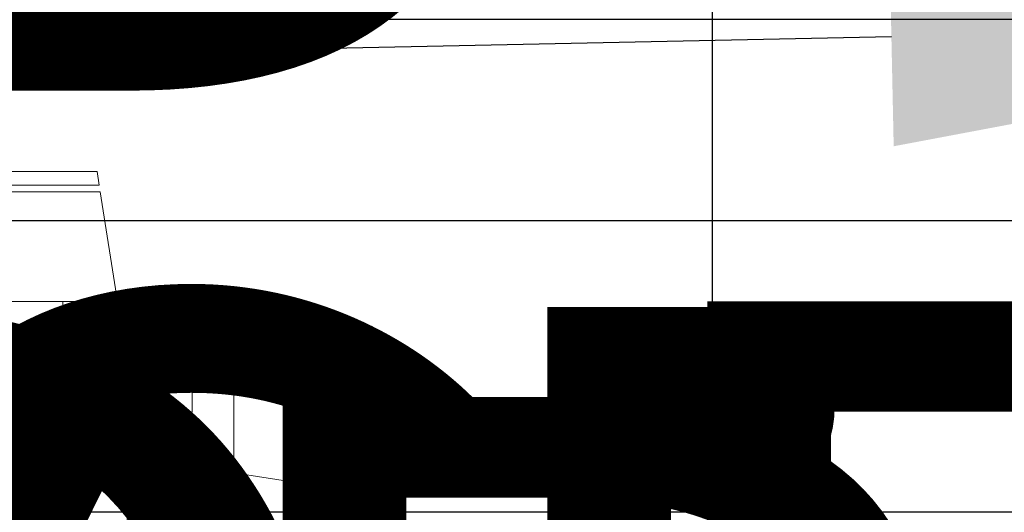
# Model space of a CAD drawing. Units: inches. Extents: x -307 to 2141, y -58 to 895.
# Tile 18 of 28: x 704 to 776, y 481 to 517. Entities that reach past the tile are written whole.
import ezdxf

# ---------------------------------------------------------------- set-up
doc = ezdxf.new("R2010")
doc.units = ezdxf.units.IN
doc.header["$MEASUREMENT"] = 0
doc.layers.add('A-ANNO-DIMS', color=2, linetype='Continuous', lineweight=18)
doc.layers.add('A-FURN', color=8, linetype='Continuous', lineweight=18)
doc.styles.get("Standard").update_dxf_attribs({"font": 'arial.ttf'})
doc.dimstyles.get("Standard").update_dxf_attribs({"dimtxt": 72, "dimasz": 48, "dimexe": 0.18, "dimexo": 0.0625, "dimgap": 0.09, "dimtad": 0, "dimtih": 1, "dimtoh": 1, "dimdec": 0, "dimrnd": 48, "dimzin": 0, "dimdsep": 46, "dimlunit": 3, "dimtxsty": 'Standard', "dimcen": 0.09, "dimadec": 0, "dimazin": 0, "dimtfac": 1, "dimtdec": 0, "dimtofl": 0, "dimtmove": 0, "dimatfit": 3, "dimfxl": 1, "dimtolj": 1, "dimtzin": 0, "dimarcsym": 0})

# ---------------------------------------------------------------- blocks, each defined once
blk = doc.blocks.new('Dining Set - 36 x 72 in.')
for p, q in [((-22, 27.5), (-22.1562, 26.50042)), ((-22, 27.5), (-6, 27.5)), ((-5.8437, 26.49966), (-6, 27.5)), ((6, 27.5), (5.8438, 26.50042)), ((6, 27.5), (22, 27.5)), ((22.1563, 26.49966), (22, 27.5)), ((-22.2343, 26.00059), (-23.4847, 17.99762)), ((-22.2304, 26), (-5.7608, 26)), ((-5.8416, 26.5), (-22.1534, 26.5)), ((-4.5152, 17.99762), (-5.7655, 25.99926)), ((5.7657, 26.00059), (4.5153, 17.99762)), ((5.7696, 26), (22.2392, 26)), ((22.1584, 26.5), (5.8466, 26.5)), ((23.4848, 17.99762), (22.2345, 25.99926)), ((36, 18), (-36, 18)), ((-36, 18), (-36, -18)), ((36, -18), (36, 18)), ((-44.0006, 8.23428), (-35.9976, 9.48474)), ((44.0006, 8.23428), (35.9976, 9.48474)), ((-45.5, 8), (-44.5004, 8.15617)), ((-45.5, 8), (-45.5, -8)), ((-44.5, -8.15843), (-44.5, 8.15338)), ((-44, 8.23041), (-44, -8.23915)), ((44, 8.23041), (44, -8.23915)), ((44.5, -8.15843), (44.5, 8.15338)), ((45.5, 8), (44.5005, 8.15617)), ((45.5, 8), (45.5, -8)), ((-44.4997, -8.15631), (-45.5, -8)), ((-35.9976, -9.48476), (-43.9993, -8.2345)), ((35.9976, -9.48476), (43.9993, -8.2345)), ((44.4997, -8.15631), (45.5, -8)), ((-36, -18), (36, -18)), ((-22.2343, -26.0006), (-23.4847, -17.99762)), ((-4.5152, -17.99762), (-5.7655, -25.99928)), ((5.7657, -26.0006), (4.5153, -17.99762)), ((23.4848, -17.99762), (22.2345, -25.99928)), ((-22.2304, -26), (-5.7608, -26)), ((-22, -27.5), (-22.1562, -26.50044)), ((-5.8416, -26.5), (-22.1534, -26.5)), ((-5.8437, -26.49967), (-6, -27.5)), ((5.7696, -26), (22.2392, -26)), ((6, -27.5), (5.8438, -26.50044)), ((22.1584, -26.5), (5.8466, -26.5)), ((22.1563, -26.49967), (22, -27.5)), ((-22, -27.5), (-6, -27.5)), ((6, -27.5), (22, -27.5))]:
    blk.add_line(p, q)
for points in [[(-36, 15), (-31.1772, 14.97754), (-26.8079, 14.91406), (-22.8538, 14.81543), (-19.276, 14.6875), (-16.0362, 14.53613), (-13.0957, 14.36718), (-10.4159, 14.18652), (-7.9583, 14), (-5.6904, 13.81315), (-3.6035, 13.63021), (-1.6954, 13.45508), (0.0365, 13.29166), (1.5945, 13.14388), (2.9811, 13.01562), (4.1988, 12.9108), (5.25, 12.83333), (6.1393, 12.78613), (6.8802, 12.76823), (7.4883, 12.77767), (7.9792, 12.8125), (8.3685, 12.87077), (8.6719, 12.95052), (8.9049, 13.0498), (9.0833, 13.16666), (9.2205, 13.29899), (9.3216, 13.44401), (9.3895, 13.59879), (9.4271, 13.76041), (9.4373, 13.92594), (9.4232, 14.09245), (9.3875, 14.257), (9.3333, 14.41666), (9.2638, 14.56917), (9.1836, 14.71484), (9.0975, 14.85465), (9.0104, 14.98958), (8.9272, 15.1206), (8.8529, 15.2487), (8.7922, 15.37483), (8.75, 15.5), (8.7305, 15.62467), (8.7344, 15.74739), (8.7617, 15.86621), (8.8125, 15.97916), (8.8867, 16.08431), (8.9844, 16.17968), (9.1055, 16.26334), (9.25, 16.33333), (9.4189, 16.38802), (9.6172, 16.42708), (9.8506, 16.45052), (10.125, 16.45833), (10.4463, 16.45052), (10.8203, 16.42708), (11.2529, 16.38802), (11.75, 16.33333), (12.3184, 16.26318), (12.9694, 16.17838), (13.7151, 16.07991), (14.5677, 15.96875), (15.5395, 15.84586), (16.6426, 15.71224), (17.8893, 15.56884), (19.2917, 15.41666), (20.859, 15.25667), (22.5879, 15.08984), (24.4721, 14.91715), (26.5052, 14.73958), (28.6809, 14.5581), (30.9929, 14.3737), (33.4347, 14.18733), (36, 14)], [(-36, 10), (-28.9766, 10.14274), (-23.1725, 10.20442), (-18.4241, 10.19775), (-14.5677, 10.13541), (-11.4399, 10.03011), (-8.877, 9.89453), (-6.7154, 9.74137), (-4.7917, 9.58333), (-2.9698, 9.43082), (-1.2246, 9.28515), (0.4415, 9.14534), (2.026, 9.01041), (3.5266, 8.87939), (4.9408, 8.7513), (6.266, 8.62516), (7.5, 8.5), (8.6411, 8.37549), (9.6914, 8.2539), (10.6538, 8.13818), (11.5312, 8.03125), (12.3267, 7.93603), (13.043, 7.85547), (13.6831, 7.79248), (14.25, 7.75), (14.7471, 7.7303), (15.1797, 7.73307), (15.5537, 7.75732), (15.875, 7.80208), (16.1494, 7.86637), (16.3828, 7.94922), (16.5811, 8.04964), (16.75, 8.16666), (16.8944, 8.29915), (17.0143, 8.44531), (17.1089, 8.60319), (17.1771, 8.77083), (17.218, 8.94629), (17.2305, 9.1276), (17.2137, 9.31282), (17.1667, 9.5), (17.0895, 9.6875), (16.987, 9.875), (16.8649, 10.0625), (16.7292, 10.25), (16.5856, 10.4375), (16.4401, 10.625), (16.2985, 10.8125), (16.1667, 11), (16.05, 11.18733), (15.9518, 11.3737), (15.8752, 11.5581), (15.8229, 11.73958), (15.798, 11.91715), (15.8034, 12.08984), (15.842, 12.25667), (15.9167, 12.41666), (16.0295, 12.56836), (16.1784, 12.70833), (16.3605, 12.83268), (16.5729, 12.9375), (16.8127, 13.01888), (17.0768, 13.07291), (17.3625, 13.0957), (17.6667, 13.08333), (17.9894, 13.03312), (18.3418, 12.94726), (18.7382, 12.82918), (19.1927, 12.68229), (19.7195, 12.51001), (20.3327, 12.31575), (21.0465, 12.10294), (21.875, 11.875), (22.8357, 11.63354), (23.959, 11.37304), (25.2786, 11.08618), (26.8282, 10.76562), (28.6414, 10.40405), (30.752, 9.99414), (33.1936, 9.52856), (36, 9)], [(-36, 5.5), (-30.7157, 5.3348), (-26.069, 5.20963), (-21.9946, 5.11767), (-18.4271, 5.05208), (-15.3009, 5.00602), (-12.5508, 4.97265), (-10.1112, 4.94515), (-7.9167, 4.91666), (-5.909, 4.88167), (-4.0586, 4.83984), (-2.3429, 4.79215), (-0.7396, 4.73958), (0.7739, 4.6831), (2.22, 4.6237), (3.6213, 4.56233), (5, 4.5), (6.373, 4.43782), (7.7344, 4.3776), (9.0723, 4.32129), (10.375, 4.27083), (11.6309, 4.22819), (12.8281, 4.19531), (13.9551, 4.17415), (15, 4.16666), (15.954, 4.17448), (16.819, 4.19791), (17.6001, 4.23698), (18.3021, 4.29166), (18.9299, 4.36198), (19.4883, 4.44791), (19.9823, 4.54948), (20.4167, 4.66666), (20.7969, 4.79899), (21.1302, 4.94401), (21.4245, 5.09879), (21.6875, 5.26041), (21.9271, 5.42594), (22.1511, 5.59245), (22.3672, 5.757), (22.5834, 5.91666), (22.8065, 6.06868), (23.0404, 6.21093), (23.2879, 6.34147), (23.5521, 6.45833), (23.8358, 6.55957), (24.142, 6.64323), (24.4735, 6.70735), (24.8334, 6.75), (25.2235, 6.76969), (25.642, 6.76692), (26.0858, 6.74267), (26.5521, 6.69791), (27.0379, 6.63362), (27.5404, 6.55078), (28.0565, 6.45036), (28.5834, 6.33333), (29.1242, 6.19987), (29.7071, 6.04687), (30.3661, 5.87044), (31.1354, 5.66666), (32.0493, 5.43164), (33.142, 5.16146), (34.4475, 4.85221), (36, 4.5)], [(-36, -1), (-30.7915, -0.6591), (-26.0195, -0.38216), (-21.6519, -0.16284), (-17.6563, 0.00521), (-14.0005, 0.12833), (-10.6523, 0.21289), (-7.5796, 0.26522), (-4.75, 0.29166), (-2.134, 0.29793), (0.2878, 0.28711), (2.5317, 0.26163), (4.6146, 0.22396), (6.5529, 0.17651), (8.3633, 0.12174), (10.0623, 0.06209), (11.6667, 0), (13.1899, -0.06201), (14.6341, -0.1211), (15.9982, -0.17432), (17.2813, -0.21875), (18.4823, -0.25147), (19.6003, -0.26953), (20.6343, -0.27002), (21.5834, -0.25), (22.4481, -0.20768), (23.2357, -0.14584), (23.9549, -0.06836), (24.6146, 0.02083), (25.2235, 0.11784), (25.7904, 0.21875), (26.3241, 0.31966), (26.8334, 0.41666), (27.3265, 0.50618), (27.8099, 0.58593), (28.2894, 0.65397), (28.7709, 0.70833), (29.2601, 0.74707), (29.763, 0.76823), (30.2855, 0.76985), (30.8334, 0.75), (31.4088, 0.70784), (31.9994, 0.64713), (32.589, 0.57275), (33.1615, 0.48958), (33.7008, 0.4025), (34.1908, 0.3164), (34.6153, 0.23616), (34.9584, 0.16666), (35.2099, 0.11165), (35.3848, 0.07031), (35.504, 0.04069), (35.5886, 0.02083), (35.6594, 0.00879), (35.7377, 0.0026), (35.8442, 0.00032), (36, 0)], [(-36, -6.5), (-27.1843, -6.31267), (-20.084, -6.1263), (-14.469, -5.9419), (-10.1094, -5.76042), (-6.7752, -5.58285), (-4.2363, -5.41016), (-2.2629, -5.24333), (-0.625, -5.08334), (0.8708, -4.93099), (2.2715, -4.78646), (3.5872, -4.64974), (4.8281, -4.52084), (6.0046, -4.39974), (7.127, -4.28646), (8.2053, -4.18099), (9.25, -4.08334), (10.2705, -3.99382), (11.2734, -3.91407), (12.2647, -3.84603), (13.25, -3.79167), (14.2354, -3.75293), (15.2266, -3.73177), (16.2295, -3.73015), (17.25, -3.75), (18.2912, -3.79248), (19.3451, -3.85547), (20.4009, -3.93604), (21.4479, -4.03125), (22.4754, -4.13819), (23.4727, -4.25391), (24.4289, -4.37549), (25.3334, -4.5), (26.1785, -4.62492), (26.9694, -4.74935), (27.7145, -4.87281), (28.4219, -4.99479), (29.1, -5.11483), (29.7572, -5.23242), (30.4016, -5.34709), (31.0417, -5.45834), (31.6837, -5.56437), (32.3262, -5.65821), (32.9658, -5.73153), (33.599, -5.77604), (34.2224, -5.78345), (34.8327, -5.74545), (35.4264, -5.65373), (36, -5.5)], [(-36, -10), (-26.4022, -9.81299), (-18.4675, -9.62891), (-11.9839, -9.45069), (-6.7396, -9.28125), (-2.5226, -9.12354), (0.8789, -8.98047), (3.6769, -8.85498), (6.0833, -8.75), (8.2767, -8.66765), (10.3021, -8.60677), (12.1712, -8.56543), (13.8958, -8.54167), (15.4876, -8.53353), (16.9583, -8.53907), (18.3197, -8.55632), (19.5834, -8.58334), (20.7616, -8.61841), (21.8685, -8.66081), (22.9188, -8.71004), (23.9271, -8.76563), (24.9081, -8.82707), (25.8763, -8.89388), (26.8465, -8.96558), (27.8334, -9.04167), (28.8474, -9.12118), (29.8828, -9.20117), (30.93, -9.27824), (31.9792, -9.34896), (33.0205, -9.40991), (34.0443, -9.45768), (35.0407, -9.48885), (36, -9.5)], [(-36, -14.5), (-30.0881, -14.33513), (-25.0332, -14.21224), (-20.7312, -14.12647), (-17.0781, -14.07292), (-13.97, -14.04671), (-11.3027, -14.04297), (-8.9724, -14.05681), (-6.875, -14.08334), (-4.9224, -14.11833), (-3.0905, -14.16016), (-1.3709, -14.20785), (0.2448, -14.26042), (1.7647, -14.3169), (3.1973, -14.3763), (4.5507, -14.43767), (5.8333, -14.5), (7.0554, -14.5621), (8.235, -14.62175), (9.3922, -14.67652), (10.5469, -14.72396), (11.7192, -14.76164), (12.929, -14.78711), (14.1965, -14.79794), (15.5417, -14.79167), (16.9933, -14.76424), (18.6152, -14.70508), (20.4804, -14.60197), (22.6615, -14.44271), (25.2312, -14.21509), (28.2624, -13.9069), (31.8277, -13.50594), (36, -13)]]:
    blk.add_lwpolyline(points)
blk = doc.blocks.new('*D26')
at = {"layer": 'A-ANNO-DIMS', "color": 0, "lineweight": -2, "transparency": 16777216}
for p, q in [((565.336, 584.202), (565.336, 572.085)), ((645.336, 584.202), (645.336, 572.085)), ((517.336, 572.265), (469.336, 572.265)), ((693.336, 572.265), (741.336, 572.265))]:
    blk.add_line(p, q, dxfattribs=at)
at = {"layer": 'A-ANNO-DIMS', "color": 0, "transparency": 16777216}
for points in [[(517.336, 580.265), (517.336, 564.265), (565.336, 572.265)], [(693.336, 580.265), (693.336, 564.265), (645.336, 572.265)]]:
    blk.add_solid(points, dxfattribs=at)
at = {"layer": 'Defpoints', "color": 0, "transparency": 16777216}
for p in [(565.336, 584.265), (645.336, 584.265), (565.336, 572.265)]:
    blk.add_point(p, dxfattribs=at)
at = {"layer": 'A-ANNO-DIMS', "color": 0, "transparency": 16777216, "insert": (178.225, 572.265), "char_height": 72, "attachment_point": 5}
blk.add_mtext('\\A1;BED 80 TYP.', dxfattribs=at)
blk = doc.blocks.new('*D29')
at = {"layer": 'A-ANNO-DIMS', "color": 0, "lineweight": -2, "transparency": 16777216}
for p, q in [((747.421, 450.871), (699.421, 450.871)), ((795.421, 433.612), (795.421, 451.051)), ((882.028, 433.612), (882.028, 451.051)), ((930.028, 450.871), (978.028, 450.871))]:
    blk.add_line(p, q, dxfattribs=at)
at = {"layer": 'A-ANNO-DIMS', "color": 0, "transparency": 16777216}
for points in [[(747.421, 458.871), (747.421, 442.871), (795.421, 450.871)], [(930.028, 458.871), (930.028, 442.871), (882.028, 450.871)]]:
    blk.add_solid(points, dxfattribs=at)
at = {"layer": 'Defpoints', "color": 0, "transparency": 16777216}
for p in [(795.421, 450.871), (795.421, 433.55), (882.028, 433.55)]:
    blk.add_point(p, dxfattribs=at)
at = {"layer": 'A-ANNO-DIMS', "color": 0, "transparency": 16777216, "insert": (647.713, 450.871), "char_height": 72, "attachment_point": 5}
blk.add_mtext('\\A1;87', dxfattribs=at)
blk = doc.blocks.new('*D30')
at = {"layer": 'A-ANNO-DIMS', "color": 0, "lineweight": -2, "transparency": 16777216}
for p, q in [((570.736, 532.833), (570.736, 580.833)), ((570.736, 580.833), (618.736, 580.833)), ((565.398, 484.833), (570.916, 484.833)), ((565.398, 448.833), (570.916, 448.833)), ((570.736, 400.833), (570.736, 352.833))]:
    blk.add_line(p, q, dxfattribs=at)
at = {"layer": 'A-ANNO-DIMS', "color": 0, "transparency": 16777216}
for points in [[(562.736, 532.833), (578.736, 532.833), (570.736, 484.833)], [(562.736, 400.833), (578.736, 400.833), (570.736, 448.833)]]:
    blk.add_solid(points, dxfattribs=at)
at = {"layer": 'Defpoints', "color": 0, "transparency": 16777216}
for p in [(565.336, 484.833), (570.736, 484.833), (565.336, 448.833)]:
    blk.add_point(p, dxfattribs=at)
at = {"layer": 'A-ANNO-DIMS', "color": 0, "transparency": 16777216, "insert": (1030.174, 580.833), "char_height": 72, "attachment_point": 5}
blk.add_mtext('\\A1;WINDOW 36 TYP.', dxfattribs=at)
blk = doc.blocks.new('*D31')
at = {"layer": 'A-ANNO-DIMS', "color": 0, "lineweight": -2, "transparency": 16777216}
for p, q in [((556.336, 448.771), (556.336, 443.253)), ((565.336, 448.771), (565.336, 443.253)), ((508.336, 443.433), (460.336, 443.433)), ((613.336, 443.433), (661.336, 443.433))]:
    blk.add_line(p, q, dxfattribs=at)
at = {"layer": 'A-ANNO-DIMS', "color": 0, "transparency": 16777216}
for points in [[(508.336, 451.433), (508.336, 435.433), (556.336, 443.433)], [(613.336, 451.433), (613.336, 435.433), (565.336, 443.433)]]:
    blk.add_solid(points, dxfattribs=at)
at = {"layer": 'Defpoints', "color": 0, "transparency": 16777216}
for p in [(556.336, 448.833), (565.336, 448.833), (565.336, 443.433)]:
    blk.add_point(p, dxfattribs=at)
at = {"layer": 'A-ANNO-DIMS', "color": 0, "transparency": 16777216, "insert": (808.692, 443.433), "char_height": 72, "attachment_point": 5}
blk.add_mtext('\\A1;9 TYP.', dxfattribs=at)
blk = doc.blocks.new('*D32')
at = {"layer": 'A-ANNO-DIMS', "color": 0, "lineweight": -2, "transparency": 16777216}
for p, q in [((813.293, 682.278), (813.293, 671.361)), ((885.293, 682.278), (885.293, 671.361)), ((765.293, 671.541), (717.293, 671.541)), ((933.293, 671.541), (981.293, 671.541))]:
    blk.add_line(p, q, dxfattribs=at)
at = {"layer": 'A-ANNO-DIMS', "color": 0, "transparency": 16777216}
for points in [[(765.293, 679.541), (765.293, 663.541), (813.293, 671.541)], [(933.293, 679.541), (933.293, 663.541), (885.293, 671.541)]]:
    blk.add_solid(points, dxfattribs=at)
at = {"layer": 'Defpoints', "color": 0, "transparency": 16777216}
for p in [(813.293, 682.341), (885.293, 682.341), (885.293, 671.541)]:
    blk.add_point(p, dxfattribs=at)
at = {"layer": 'A-ANNO-DIMS', "color": 0, "transparency": 16777216, "insert": (1392.731, 671.541), "char_height": 72, "attachment_point": 5}
blk.add_mtext('\\A1;WINDOW 72 TYP.', dxfattribs=at)
blk = doc.blocks.new('*D35')
at = {"layer": 'A-ANNO-DIMS', "color": 0, "lineweight": -2, "transparency": 16777216}
for p, q in [((859.336, 453.769), (811.336, 453.769)), ((907.336, 443.029), (907.336, 453.949)), ((916.336, 443.029), (916.336, 453.949)), ((964.336, 453.769), (1012.336, 453.769))]:
    blk.add_line(p, q, dxfattribs=at)
at = {"layer": 'A-ANNO-DIMS', "color": 0, "transparency": 16777216}
for points in [[(859.336, 461.769), (859.336, 445.769), (907.336, 453.769)], [(964.336, 461.769), (964.336, 445.769), (916.336, 453.769)]]:
    blk.add_solid(points, dxfattribs=at)
at = {"layer": 'Defpoints', "color": 0, "transparency": 16777216}
for p in [(907.336, 453.769), (907.336, 442.967), (916.336, 442.967)]:
    blk.add_point(p, dxfattribs=at)
at = {"layer": 'A-ANNO-DIMS', "color": 0, "transparency": 16777216, "insert": (663.98, 453.769), "char_height": 72, "attachment_point": 5}
blk.add_mtext('\\A1;9 TYP.', dxfattribs=at)
blk = doc.blocks.new('*D36')
at = {"layer": 'A-ANNO-DIMS', "color": 0, "lineweight": -2, "transparency": 16777216}
for p, q in [((871.707, 562.404), (871.761, 610.404)), ((876.548, 514.399), (871.474, 514.405)), ((876.511, 481.353), (871.437, 481.358)), ((871.563, 433.358), (871.509, 385.358)), ((871.509, 385.358), (823.509, 385.358))]:
    blk.add_line(p, q, dxfattribs=at)
at = {"layer": 'A-ANNO-DIMS', "color": 0, "transparency": 16777216}
for points in [[(863.707, 562.413), (879.707, 562.395), (871.654, 514.404)], [(863.563, 433.367), (879.563, 433.349), (871.617, 481.358)]]:
    blk.add_solid(points, dxfattribs=at)
at = {"layer": 'Defpoints', "color": 0, "transparency": 16777216}
for p in [(876.611, 514.399), (871.617, 481.358), (876.574, 481.353)]:
    blk.add_point(p, dxfattribs=at)
at = {"layer": 'A-ANNO-DIMS', "color": 0, "transparency": 16777216, "insert": (548.95, 385.358), "char_height": 72, "attachment_point": 5}
blk.add_mtext('\\A1;WC 33 TYP.', dxfattribs=at)
blk = doc.blocks.new('*D37')
at = {"layer": 'A-ANNO-DIMS', "color": 0, "lineweight": -2, "transparency": 16777216}
for p, q in [((828.616, 519.409), (780.616, 519.463)), ((876.611, 514.461), (876.616, 519.536)), ((897.611, 514.438), (897.616, 519.512)), ((945.616, 519.279), (993.616, 519.225))]:
    blk.add_line(p, q, dxfattribs=at)
at = {"layer": 'A-ANNO-DIMS', "color": 0, "transparency": 16777216}
for points in [[(828.625, 527.409), (828.607, 511.409), (876.616, 519.356)], [(945.625, 527.279), (945.607, 511.279), (897.616, 519.332)]]:
    blk.add_solid(points, dxfattribs=at)
at = {"layer": 'Defpoints', "color": 0, "transparency": 16777216}
for p in [(876.616, 519.356), (876.611, 514.399), (897.611, 514.375)]:
    blk.add_point(p, dxfattribs=at)
at = {"layer": 'A-ANNO-DIMS', "color": 0, "transparency": 16777216, "insert": (604.676, 519.463), "char_height": 72, "attachment_point": 5}
blk.add_mtext('\\A1;21 TYP.', dxfattribs=at)
blk = doc.blocks.new('*D42')
at = {"layer": 'A-ANNO-DIMS', "color": 0, "lineweight": -2, "transparency": 16777216}
for p, q in [((880.259, 543.859), (928.248, 544.868)), ((822.302, 541.203), (822.268, 542.82)), ((832.299, 541.413), (832.265, 543.03)), ((774.282, 541.631), (726.293, 540.622))]:
    blk.add_line(p, q, dxfattribs=at)
at = {"layer": 'A-ANNO-DIMS', "color": 0, "transparency": 16777216}
for points in [[(880.09, 551.857), (880.427, 535.861), (832.269, 542.85)], [(774.114, 549.629), (774.45, 533.633), (822.271, 542.64)]]:
    blk.add_solid(points, dxfattribs=at)
at = {"layer": 'Defpoints', "color": 0, "transparency": 16777216}
for p in [(832.269, 542.85), (832.301, 541.35), (822.303, 541.14)]:
    blk.add_point(p, dxfattribs=at)
at = {"layer": 'A-ANNO-DIMS', "color": 0, "transparency": 16777216, "insert": (1192.886, 544.868), "char_height": 72, "attachment_point": 5}
blk.add_mtext('\\A1;FAUCET 10', dxfattribs=at)
blk = doc.blocks.new('*D43')
at = {"layer": 'A-ANNO-DIMS', "color": 0, "lineweight": -2, "transparency": 16777216}
for p, q in [((818.785, 637.088), (770.785, 637.088)), ((819.794, 589.098), (818.785, 637.088)), ((822.24, 541.139), (820.623, 541.105)), ((822.377, 534.64), (820.76, 534.606)), ((821.949, 486.621), (822.958, 438.631))]:
    blk.add_line(p, q, dxfattribs=at)
at = {"layer": 'A-ANNO-DIMS', "color": 0, "transparency": 16777216}
for points in [[(827.792, 589.266), (811.796, 588.93), (820.803, 541.109)], [(829.947, 486.789), (813.951, 486.453), (820.94, 534.61)]]:
    blk.add_solid(points, dxfattribs=at)
at = {"layer": 'Defpoints', "color": 0, "transparency": 16777216}
for p in [(820.803, 541.109), (822.303, 541.14), (822.44, 534.642)]:
    blk.add_point(p, dxfattribs=at)
at = {"layer": 'A-ANNO-DIMS', "color": 0, "transparency": 16777216, "insert": (747.391, 637.088), "char_height": 72, "attachment_point": 5}
blk.add_mtext('\\A1;7', dxfattribs=at)
blk = doc.blocks.new('*D44')
at = {"layer": 'A-ANNO-DIMS', "color": 0, "lineweight": -2, "transparency": 16777216}
for p, q in [((839.872, 521.223), (839.952, 517.424)), ((815.327, 520.707), (815.406, 516.907)), ((887.938, 518.613), (935.927, 519.622)), ((767.413, 516.078), (719.424, 515.069))]:
    blk.add_line(p, q, dxfattribs=at)
at = {"layer": 'A-ANNO-DIMS', "color": 0, "transparency": 16777216}
for points in [[(887.769, 526.611), (888.106, 510.614), (839.948, 517.604)], [(767.245, 524.076), (767.581, 508.08), (815.403, 517.087)]]:
    blk.add_solid(points, dxfattribs=at)
at = {"layer": 'Defpoints', "color": 0, "transparency": 16777216}
for p in [(839.871, 521.285), (815.325, 520.769), (839.948, 517.604)]:
    blk.add_point(p, dxfattribs=at)
at = {"layer": 'A-ANNO-DIMS', "color": 0, "transparency": 16777216, "insert": (1151.157, 519.622), "char_height": 72, "attachment_point": 5}
blk.add_mtext('\\A1;BASIN 25', dxfattribs=at)
blk = doc.blocks.new('*D45')
at = {"layer": 'A-ANNO-DIMS', "color": 0, "lineweight": -2, "transparency": 16777216}
for p, q in [((841.111, 637.474), (793.111, 637.474)), ((842.12, 589.484), (841.111, 637.474)), ((839.51, 541.419), (843.309, 541.499)), ((839.933, 521.287), (843.732, 521.367)), ((844.562, 473.373), (845.571, 425.384))]:
    blk.add_line(p, q, dxfattribs=at)
at = {"layer": 'A-ANNO-DIMS', "color": 0, "transparency": 16777216}
for points in [[(850.118, 589.652), (834.122, 589.316), (843.129, 541.495)], [(852.56, 473.542), (836.563, 473.205), (843.553, 521.363)]]:
    blk.add_solid(points, dxfattribs=at)
at = {"layer": 'Defpoints', "color": 0, "transparency": 16777216}
for p in [(839.447, 541.417), (843.129, 541.495), (839.871, 521.285)]:
    blk.add_point(p, dxfattribs=at)
at = {"layer": 'A-ANNO-DIMS', "color": 0, "transparency": 16777216, "insert": (740.961, 637.474), "char_height": 72, "attachment_point": 5}
blk.add_mtext('\\A1;20', dxfattribs=at)
blk = doc.blocks.new('*D46')
at = {"layer": 'A-ANNO-DIMS', "color": 0, "lineweight": -2, "transparency": 16777216}
for p, q in [((801.413, 645.783), (801.413, 642.516)), ((822.413, 645.783), (822.413, 642.516)), ((753.413, 642.696), (705.413, 642.696)), ((870.413, 642.696), (918.413, 642.696))]:
    blk.add_line(p, q, dxfattribs=at)
at = {"layer": 'A-ANNO-DIMS', "color": 0, "transparency": 16777216}
for points in [[(753.413, 650.696), (753.413, 634.696), (801.413, 642.696)], [(870.413, 650.696), (870.413, 634.696), (822.413, 642.696)]]:
    blk.add_solid(points, dxfattribs=at)
at = {"layer": 'Defpoints', "color": 0, "transparency": 16777216}
for p in [(801.413, 645.846), (822.413, 645.846), (822.413, 642.696)]:
    blk.add_point(p, dxfattribs=at)
at = {"layer": 'A-ANNO-DIMS', "color": 0, "transparency": 16777216, "insert": (1282.702, 642.696), "char_height": 72, "attachment_point": 5}
blk.add_mtext('\\A1;DESK CHAIR 21', dxfattribs=at)
blk = doc.blocks.new('*D52')
at = {"layer": 'A-ANNO-DIMS', "color": 0, "lineweight": -2, "transparency": 16777216}
for p, q in [((660.208, 554.249), (660.208, 602.249)), ((673.796, 506.249), (660.028, 506.249)), ((673.796, 415.249), (660.028, 415.249)), ((660.208, 367.249), (660.208, 319.249))]:
    blk.add_line(p, q, dxfattribs=at)
at = {"layer": 'A-ANNO-DIMS', "color": 0, "transparency": 16777216}
for points in [[(652.208, 554.249), (668.208, 554.249), (660.208, 506.249)], [(652.208, 367.249), (668.208, 367.249), (660.208, 415.249)]]:
    blk.add_solid(points, dxfattribs=at)
at = {"layer": 'Defpoints', "color": 0, "transparency": 16777216}
for p in [(673.858, 506.249), (660.208, 415.249), (673.858, 415.249)]:
    blk.add_point(p, dxfattribs=at)
at = {"layer": 'A-ANNO-DIMS', "color": 0, "transparency": 16777216, "insert": (660.208, 460.749), "char_height": 72, "attachment_point": 5}
blk.add_mtext('\\A1;DINING SET 91', dxfattribs=at)
blk = doc.blocks.new('*D54')
at = {"layer": 'A-ANNO-DIMS', "color": 0, "lineweight": -2, "transparency": 16777216}
for p, q in [((605.336, 412.349), (605.336, 460.349)), ((605.336, 460.349), (653.336, 460.349)), ((596.398, 364.349), (605.516, 364.349)), ((596.398, 304.349), (605.516, 304.349)), ((605.336, 256.349), (605.336, 208.349))]:
    blk.add_line(p, q, dxfattribs=at)
at = {"layer": 'A-ANNO-DIMS', "color": 0, "transparency": 16777216}
for points in [[(597.336, 412.349), (613.336, 412.349), (605.336, 364.349)], [(597.336, 256.349), (613.336, 256.349), (605.336, 304.349)]]:
    blk.add_solid(points, dxfattribs=at)
at = {"layer": 'Defpoints', "color": 0, "transparency": 16777216}
for p in [(596.336, 364.349), (605.336, 364.349), (596.336, 304.349)]:
    blk.add_point(p, dxfattribs=at)
at = {"layer": 'A-ANNO-DIMS', "color": 0, "transparency": 16777216, "insert": (854.004, 460.349), "char_height": 72, "attachment_point": 5}
blk.add_mtext('\\A1;DESK 60', dxfattribs=at)
blk = doc.blocks.new('*D62')
at = {"layer": 'A-ANNO-DIMS', "color": 0, "lineweight": -2, "transparency": 16777216}
for p, q in [((556.336, 691.403), (556.336, 722.725)), ((604.336, 722.545), (656.854, 722.545)), ((868.336, 722.545), (815.817, 722.545)), ((916.336, 490.966), (916.336, 722.725))]:
    blk.add_line(p, q, dxfattribs=at)
at = {"layer": 'A-ANNO-DIMS', "color": 0, "transparency": 16777216}
for points in [[(604.336, 730.545), (604.336, 714.545), (556.336, 722.545)], [(868.336, 730.545), (868.336, 714.545), (916.336, 722.545)]]:
    blk.add_solid(points, dxfattribs=at)
at = {"layer": 'Defpoints', "color": 0, "transparency": 16777216}
for p in [(916.336, 722.545), (556.336, 691.341), (916.336, 490.903)]:
    blk.add_point(p, dxfattribs=at)
at = {"layer": 'A-ANNO-DIMS', "color": 0, "transparency": 16777216, "insert": (736.336, 722.545), "char_height": 72, "attachment_point": 5}
blk.add_mtext('\\A1;360', dxfattribs=at)
blk = doc.blocks.new('*D63')
at = {"layer": 'A-ANNO-DIMS', "color": 0, "lineweight": -2, "transparency": 16777216}
for p, q in [((916.398, 691.341), (947.72, 691.341)), ((947.54, 643.341), (947.54, 416.192)), ((947.54, 115.341), (947.54, 342.49)), ((704.684, 67.341), (947.72, 67.341))]:
    blk.add_line(p, q, dxfattribs=at)
at = {"layer": 'A-ANNO-DIMS', "color": 0, "transparency": 16777216}
for points in [[(939.54, 643.341), (955.54, 643.341), (947.54, 691.341)], [(939.54, 115.341), (955.54, 115.341), (947.54, 67.341)]]:
    blk.add_solid(points, dxfattribs=at)
at = {"layer": 'Defpoints', "color": 0, "transparency": 16777216}
for p in [(916.336, 691.341), (704.621, 67.341), (947.54, 67.341)]:
    blk.add_point(p, dxfattribs=at)
at = {"layer": 'A-ANNO-DIMS', "color": 0, "transparency": 16777216, "insert": (947.54, 379.341), "char_height": 72, "attachment_point": 5}
blk.add_mtext('\\A1;624', dxfattribs=at)
blk = doc.blocks.new('*D68')
at = {"layer": 'A-ANNO-DIMS', "color": 0, "lineweight": -2, "transparency": 16777216}
for p, q in [((525.132, 586.341), (525.132, 634.341)), ((525.132, 634.341), (573.132, 634.341)), ((565.273, 538.341), (524.952, 538.341)), ((556.273, 484.833), (524.952, 484.833)), ((525.132, 436.833), (525.132, 388.833))]:
    blk.add_line(p, q, dxfattribs=at)
at = {"layer": 'A-ANNO-DIMS', "color": 0, "transparency": 16777216}
for points in [[(517.132, 586.341), (533.132, 586.341), (525.132, 538.341)], [(517.132, 436.833), (533.132, 436.833), (525.132, 484.833)]]:
    blk.add_solid(points, dxfattribs=at)
at = {"layer": 'Defpoints', "color": 0, "transparency": 16777216}
for p in [(525.132, 538.341), (565.336, 538.341), (556.336, 484.833)]:
    blk.add_point(p, dxfattribs=at)
at = {"layer": 'A-ANNO-DIMS', "color": 0, "transparency": 16777216, "insert": (687.754, 634.341), "char_height": 72, "attachment_point": 5}
blk.add_mtext('\\A1;53.51', dxfattribs=at)
blk = doc.blocks.new('*D78')
at = {"layer": 'A-ANNO-DIMS', "color": 0, "lineweight": -2, "transparency": 16777216}
for p, q in [((947.53984, 730.340828), (947.53984, 778.340828)), ((778.39834, 682.340828), (947.71984, 682.340828)), ((730.39834, 598.340828), (947.71984, 598.340828)), ((947.53984, 550.340828), (947.53984, 502.340828))]:
    blk.add_line(p, q, dxfattribs=at)
at = {"layer": 'A-ANNO-DIMS', "color": 0, "transparency": 16777216}
for points in [[(939.53984, 730.340828), (955.53984, 730.340828), (947.53984, 682.340828)], [(939.53984, 550.340828), (955.53984, 550.340828), (947.53984, 598.340828)]]:
    blk.add_solid(points, dxfattribs=at)
at = {"layer": 'Defpoints', "color": 0, "transparency": 16777216}
for p in [(778.33584, 682.340828), (947.53984, 682.340828), (730.33584, 598.340828)]:
    blk.add_point(p, dxfattribs=at)
at = {"layer": 'A-ANNO-DIMS', "color": 0, "transparency": 16777216, "insert": (947.53984, 640.340828), "char_height": 72, "attachment_point": 5}
blk.add_mtext('\\A1;84', dxfattribs=at)
blk = doc.blocks.new('*D82')
at = {"layer": 'A-ANNO-DIMS', "color": 0, "lineweight": -2, "transparency": 16777216}
for p, q in [((525.132, 565.341), (525.132, 613.341)), ((525.132, 613.341), (573.132, 613.341)), ((802.273, 517.341), (524.952, 517.341)), ((802.273, 481.341), (524.952, 481.341)), ((525.132, 433.341), (525.132, 385.341))]:
    blk.add_line(p, q, dxfattribs=at)
at = {"layer": 'A-ANNO-DIMS', "color": 0, "transparency": 16777216}
for points in [[(517.132, 565.341), (533.132, 565.341), (525.132, 517.341)], [(517.132, 433.341), (533.132, 433.341), (525.132, 481.341)]]:
    blk.add_solid(points, dxfattribs=at)
at = {"layer": 'Defpoints', "color": 0, "transparency": 16777216}
for p in [(525.132, 517.341), (802.336, 517.341), (802.336, 481.341)]:
    blk.add_point(p, dxfattribs=at)
at = {"layer": 'A-ANNO-DIMS', "color": 0, "transparency": 16777216, "insert": (624.742, 613.341), "char_height": 72, "attachment_point": 5}
blk.add_mtext('\\A1;36', dxfattribs=at)
blk = doc.blocks.new('*D83')
at = {"layer": 'A-ANNO-DIMS', "color": 0, "lineweight": -2, "transparency": 16777216}
for p, q in [((947.54, 538.903), (947.54, 586.903)), ((916.398, 490.903), (947.72, 490.903)), ((907.398, 481.341), (947.72, 481.341)), ((947.54, 433.341), (947.54, 385.341)), ((947.54, 385.341), (899.54, 385.341))]:
    blk.add_line(p, q, dxfattribs=at)
at = {"layer": 'A-ANNO-DIMS', "color": 0, "transparency": 16777216}
for points in [[(939.54, 538.903), (955.54, 538.903), (947.54, 490.903)], [(939.54, 433.341), (955.54, 433.341), (947.54, 481.341)]]:
    blk.add_solid(points, dxfattribs=at)
at = {"layer": 'Defpoints', "color": 0, "transparency": 16777216}
for p in [(916.336, 490.903), (907.336, 481.341), (947.54, 481.341)]:
    blk.add_point(p, dxfattribs=at)
at = {"layer": 'A-ANNO-DIMS', "color": 0, "transparency": 16777216, "insert": (777.968, 385.341), "char_height": 72, "attachment_point": 5}
blk.add_mtext('\\A1;9.563', dxfattribs=at)
blk = doc.blocks.new('*D88')
at = {"layer": 'A-ANNO-DIMS', "color": 0, "lineweight": -2, "transparency": 16777216}
for p, q in [((517.33584, 722.544828), (469.33584, 722.544828)), ((565.33584, 295.403328), (565.33584, 722.724828)), ((754.33584, 271.403328), (754.33584, 722.724828)), ((802.33584, 722.544828), (850.33584, 722.544828))]:
    blk.add_line(p, q, dxfattribs=at)
at = {"layer": 'A-ANNO-DIMS', "color": 0, "transparency": 16777216}
for points in [[(517.33584, 730.544828), (517.33584, 714.544828), (565.33584, 722.544828)], [(802.33584, 730.544828), (802.33584, 714.544828), (754.33584, 722.544828)]]:
    blk.add_solid(points, dxfattribs=at)
at = {"layer": 'Defpoints', "color": 0, "transparency": 16777216}
for p in [(754.33584, 722.544828), (565.33584, 295.340828), (754.33584, 271.340828)]:
    blk.add_point(p, dxfattribs=at)
at = {"layer": 'A-ANNO-DIMS', "color": 0, "transparency": 16777216, "insert": (659.83584, 722.544828), "char_height": 72, "attachment_point": 5}
blk.add_mtext('\\A1;189', dxfattribs=at)
blk = doc.blocks.new('*D95')
at = {"layer": 'A-ANNO-DIMS', "color": 0, "lineweight": -2, "transparency": 16777216}
for p, q in [((947.54, 577.341), (947.54, 625.341)), ((947.54, 625.341), (995.54, 625.341)), ((629.898, 529.341), (947.72, 529.341)), ((629.898, 502.663), (947.72, 502.663)), ((947.54, 454.663), (947.54, 406.663))]:
    blk.add_line(p, q, dxfattribs=at)
at = {"layer": 'A-ANNO-DIMS', "color": 0, "transparency": 16777216}
for points in [[(939.54, 577.341), (955.54, 577.341), (947.54, 529.341)], [(939.54, 454.663), (955.54, 454.663), (947.54, 502.663)]]:
    blk.add_solid(points, dxfattribs=at)
at = {"layer": 'Defpoints', "color": 0, "transparency": 16777216}
for p in [(629.836, 529.341), (947.54, 529.341), (629.836, 502.663)]:
    blk.add_point(p, dxfattribs=at)
at = {"layer": 'A-ANNO-DIMS', "color": 0, "transparency": 16777216, "insert": (1117.799, 625.341), "char_height": 72, "attachment_point": 5}
blk.add_mtext('\\A1;26.68', dxfattribs=at)
blk = doc.blocks.new('*D97')
at = {"layer": 'A-ANNO-DIMS', "color": 0, "lineweight": -2, "transparency": 16777216}
for p, q in [((947.54, 637.341), (947.54, 685.341)), ((947.54, 685.341), (995.54, 685.341)), ((685.398, 589.341), (947.72, 589.341)), ((685.398, 538.341), (947.72, 538.341)), ((947.54, 490.341), (947.54, 442.341))]:
    blk.add_line(p, q, dxfattribs=at)
at = {"layer": 'A-ANNO-DIMS', "color": 0, "transparency": 16777216}
for points in [[(939.54, 637.341), (955.54, 637.341), (947.54, 589.341)], [(939.54, 490.341), (955.54, 490.341), (947.54, 538.341)]]:
    blk.add_solid(points, dxfattribs=at)
at = {"layer": 'Defpoints', "color": 0, "transparency": 16777216}
for p in [(685.336, 589.341), (947.54, 589.341), (685.336, 538.341)]:
    blk.add_point(p, dxfattribs=at)
at = {"layer": 'A-ANNO-DIMS', "color": 0, "transparency": 16777216, "insert": (1040.249, 685.341), "char_height": 72, "attachment_point": 5}
blk.add_mtext('\\A1;51', dxfattribs=at)
blk = doc.blocks.new('*D98')
at = {"layer": 'A-ANNO-DIMS', "color": 0, "lineweight": -2, "transparency": 16777216}
for p, q in [((525.132, 637.341), (525.132, 685.341)), ((525.132, 685.341), (573.132, 685.341)), ((787.273, 589.341), (524.952, 589.341)), ((787.273, 550.341), (524.952, 550.341)), ((525.132, 502.341), (525.132, 454.341))]:
    blk.add_line(p, q, dxfattribs=at)
at = {"layer": 'A-ANNO-DIMS', "color": 0, "transparency": 16777216}
for points in [[(517.132, 637.341), (533.132, 637.341), (525.132, 589.341)], [(517.132, 502.341), (533.132, 502.341), (525.132, 550.341)]]:
    blk.add_solid(points, dxfattribs=at)
at = {"layer": 'Defpoints', "color": 0, "transparency": 16777216}
for p in [(525.132, 589.341), (787.336, 589.341), (787.336, 550.341)]:
    blk.add_point(p, dxfattribs=at)
at = {"layer": 'A-ANNO-DIMS', "color": 0, "transparency": 16777216, "insert": (624.84, 685.341), "char_height": 72, "attachment_point": 5}
blk.add_mtext('\\A1;39', dxfattribs=at)
blk = doc.blocks.new('*D107')
at = {"layer": 'A-ANNO-DIMS', "color": 0, "lineweight": -2, "transparency": 16777216}
for p, q in [((517.336, 722.545), (469.336, 722.545)), ((565.336, 409.403), (565.336, 722.725)), ((589.339, 409.403), (589.339, 722.725)), ((637.339, 722.545), (685.339, 722.545))]:
    blk.add_line(p, q, dxfattribs=at)
at = {"layer": 'A-ANNO-DIMS', "color": 0, "transparency": 16777216}
for points in [[(517.336, 730.545), (517.336, 714.545), (565.336, 722.545)], [(637.339, 730.545), (637.339, 714.545), (589.339, 722.545)]]:
    blk.add_solid(points, dxfattribs=at)
at = {"layer": 'Defpoints', "color": 0, "transparency": 16777216}
for p in [(589.339, 722.545), (565.336, 409.341), (589.339, 409.341)]:
    blk.add_point(p, dxfattribs=at)
at = {"layer": 'A-ANNO-DIMS', "color": 0, "transparency": 16777216, "insert": (835.495, 722.545), "char_height": 72, "attachment_point": 5}
blk.add_mtext('\\A1;24.003', dxfattribs=at)
blk = doc.blocks.new('*D108')
at = {"layer": 'A-ANNO-DIMS', "color": 0, "lineweight": -2, "transparency": 16777216}
for p, q in [((947.54, 550.663), (947.54, 598.663)), ((589.402, 502.663), (947.72, 502.663)), ((589.402, 409.341), (947.72, 409.341)), ((947.54, 361.341), (947.54, 313.341))]:
    blk.add_line(p, q, dxfattribs=at)
at = {"layer": 'A-ANNO-DIMS', "color": 0, "transparency": 16777216}
for points in [[(939.54, 550.663), (955.54, 550.663), (947.54, 502.663)], [(939.54, 361.341), (955.54, 361.341), (947.54, 409.341)]]:
    blk.add_solid(points, dxfattribs=at)
at = {"layer": 'Defpoints', "color": 0, "transparency": 16777216}
for p in [(589.339, 502.663), (947.54, 502.663), (589.339, 409.341)]:
    blk.add_point(p, dxfattribs=at)
at = {"layer": 'A-ANNO-DIMS', "color": 0, "transparency": 16777216, "insert": (947.54, 456.002), "char_height": 72, "attachment_point": 5}
blk.add_mtext('\\A1;93.32', dxfattribs=at)

msp = doc.modelspace()

# ---------------------------------------------------------------- block references
at = {"layer": 'A-FURN', "rotation": 270}
msp.add_blockref('Dining Set - 36 x 72 in.', (701.3583, 460.7485), dxfattribs=at)

# ---------------------------------------------------------------- dimensions: what is measured, and where the dimension line sits
at = {"layer": 'A-ANNO-DIMS'}
for base, p1, p2, text, picture, middle in [((885.2934, 671.5408), (813.2934, 682.3408), (885.2934, 682.3408), 'WINDOW <> TYP.', '*D32', (1392.7312, 671.5408)), ((822.4132, 642.696), (801.4132, 645.846), (822.4132, 645.846), 'DESK CHAIR <>', '*D46', (1282.7024, 642.696)), ((565.3358, 443.4333), (556.3358, 448.8333), (565.3358, 448.8333), '<> TYP.', '*D31', (808.6919, 443.4333))]:
    dim = msp.add_linear_dim(base=base, p1=p1, p2=p2, text=text, dimstyle='Standard', override={"dimdec": 0, "dimlfac": 1, "dimrnd": 0, "dimzin": 0, "dimdsep": 46, "dimlunit": 2}, dxfattribs=at)
    dim.commit()
    dim.dimension.update_dxf_attribs({"geometry": picture, "text_midpoint": middle})
for base, p1, p2, angle, override, picture, middle in [((947.5398, 682.3408), (730.3358, 598.3408), (778.3358, 682.3408), 90, {"dimdec": 0, "dimlfac": 1, "dimrnd": 0, "dimzin": 0, "dimdsep": 46, "dimlunit": 2}, '*D78', (947.5398, 640.3408)), ((525.1318, 589.3408), (787.3358, 550.3408), (787.3358, 589.3408), 90, {"dimdec": 0, "dimlfac": 1, "dimrnd": 0, "dimzin": 0, "dimdsep": 46, "dimlunit": 2}, '*D98', (624.8398, 685.3408)), ((947.5398, 589.3408), (685.3358, 538.3408), (685.3358, 589.3408), 90, {"dimdec": 0, "dimlfac": 1, "dimrnd": 0, "dimzin": 0, "dimdsep": 46, "dimlunit": 2}, '*D97', (1040.2492, 685.3408)), ((947.5398, 67.3408), (916.3358, 691.3408), (704.6211, 67.3408), 90, {"dimdec": 0, "dimlfac": 1, "dimrnd": 0, "dimzin": 0, "dimdsep": 46, "dimlunit": 2}, '*D63', (947.5398, 379.3408)), ((843.1292, 541.4949), (839.8707, 521.2853), (839.4474, 541.4175), 91.204628, {"dimdec": 0, "dimlfac": 1, "dimrnd": 0, "dimzin": 0, "dimdsep": 46, "dimlunit": 2}, '*D45', (740.961, 637.4737)), ((820.8033, 541.1087), (822.4396, 534.6416), (822.3029, 541.1403), 91.204628, {"dimdec": 0, "dimlfac": 1, "dimrnd": 0, "dimzin": 0, "dimdsep": 46, "dimlunit": 2}, '*D43', (747.3908, 637.0875)), ((525.1318, 538.3408), (556.3358, 484.8333), (565.3358, 538.3408), 90, {"dimdec": 2, "dimlfac": 1, "dimrnd": 0, "dimzin": 0, "dimdsep": 46, "dimlunit": 2}, '*D68', (687.7539, 634.3408)), ((947.5398, 529.3408), (629.8358, 502.6632), (629.8358, 529.3408), 90, {"dimdec": 2, "dimlfac": 1, "dimrnd": 0, "dimzin": 0, "dimdsep": 46, "dimlunit": 2}, '*D95', (1117.799, 625.3408)), ((525.1318, 517.3408), (802.3358, 481.3408), (802.3358, 517.3408), 90, {"dimdec": 0, "dimlfac": 1, "dimrnd": 0, "dimzin": 0, "dimdsep": 46, "dimlunit": 2}, '*D82', (624.7416, 613.3408)), ((947.5398, 502.6632), (589.339, 409.3408), (589.339, 502.6632), 90, {"dimdec": 2, "dimlfac": 1, "dimrnd": 0, "dimzin": 0, "dimdsep": 46, "dimlunit": 2}, '*D108', (947.5398, 456.002)), ((947.5398, 481.3408), (916.3358, 490.9034), (907.3358, 481.3408), 90, {"dimdec": 3, "dimlfac": 1, "dimrnd": 0, "dimzin": 0, "dimdsep": 46, "dimlunit": 2}, '*D83', (777.9683, 385.3408)), ((795.4208, 450.8711), (882.0282, 433.5496), (795.4208, 433.5496), 180, {"dimdec": 0, "dimlfac": 1, "dimrnd": 0, "dimzin": 0, "dimdsep": 46, "dimlunit": 2}, '*D29', (647.7128, 450.8711))]:
    dim = msp.add_linear_dim(base=base, p1=p1, p2=p2, angle=angle, dimstyle='Standard', override=override, dxfattribs=at)
    dim.commit()
    dim.dimension.update_dxf_attribs({"geometry": picture, "text_midpoint": middle})
for base, p1, p2, override, picture, middle in [((754.3358, 722.5448), (565.3358, 295.3408), (754.3358, 271.3408), {"dimdec": 0, "dimlfac": 1, "dimrnd": 0, "dimzin": 0, "dimdsep": 46, "dimlunit": 2}, '*D88', (659.8358, 722.5448)), ((589.339, 722.5448), (565.3358, 409.3408), (589.339, 409.3408), {"dimdec": 3, "dimlfac": 1, "dimrnd": 0, "dimzin": 0, "dimdsep": 46, "dimlunit": 2}, '*D107', (835.4945, 722.5448)), ((916.3358, 722.5448), (556.3358, 691.3408), (916.3358, 490.9034), {"dimdec": 0, "dimlfac": 1, "dimrnd": 0, "dimzin": 0, "dimdsep": 46, "dimlunit": 2}, '*D62', (736.3358, 722.5448))]:
    dim = msp.add_linear_dim(base=base, p1=p1, p2=p2, dimstyle='Standard', override=override, dxfattribs=at)
    dim.commit()
    dim.dimension.update_dxf_attribs({"geometry": picture, "text_midpoint": middle})
for base, p1, p2, angle, text, picture, middle in [((570.7358, 484.8333), (565.3358, 448.8333), (565.3358, 484.8333), 90, 'WINDOW <> TYP.', '*D30', (1030.1737, 580.8333)), ((565.3358, 572.2648), (645.3359, 584.2648), (565.3358, 584.2648), 180, 'BED <> TYP.', '*D26', (178.2254, 572.2648)), ((832.2692, 542.8502), (822.3029, 541.1403), (832.3007, 541.3505), 1.204628, 'FAUCET <>', '*D42', (1192.8864, 544.8684)), ((660.2083, 415.2485), (673.8583, 506.2485), (673.8583, 415.2485), 270, 'DINING SET <>', '*D52', (660.2083, 460.7485)), ((876.6162, 519.3557), (897.6106, 514.3753), (876.6106, 514.3988), 179.935892, '<> TYP.', '*D37', (604.6763, 519.4631)), ((839.9481, 517.6035), (815.3253, 520.7692), (839.8707, 521.2853), 1.204628, 'BASIN <>', '*D44', (1151.1574, 519.6217)), ((871.6167, 481.3581), (876.6106, 514.3988), (876.5736, 481.3526), 269.935892, 'WC <> TYP.', '*D36', (548.95, 385.3582)), ((605.3358, 364.3488), (596.3358, 304.3488), (596.3358, 364.3488), 90, 'DESK <>', '*D54', (854.0043, 460.3488)), ((907.3358, 453.7692), (916.3358, 442.9669), (907.3358, 442.9669), 180, '<> TYP.', '*D35', (663.9798, 453.7692))]:
    dim = msp.add_linear_dim(base=base, p1=p1, p2=p2, angle=angle, text=text, dimstyle='Standard', override={"dimdec": 0, "dimlfac": 1, "dimrnd": 0, "dimzin": 0, "dimdsep": 46, "dimlunit": 2}, dxfattribs=at)
    dim.commit()
    dim.dimension.update_dxf_attribs({"geometry": picture, "text_midpoint": middle})

doc.saveas('drawing.dxf')
